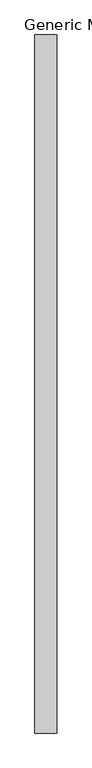
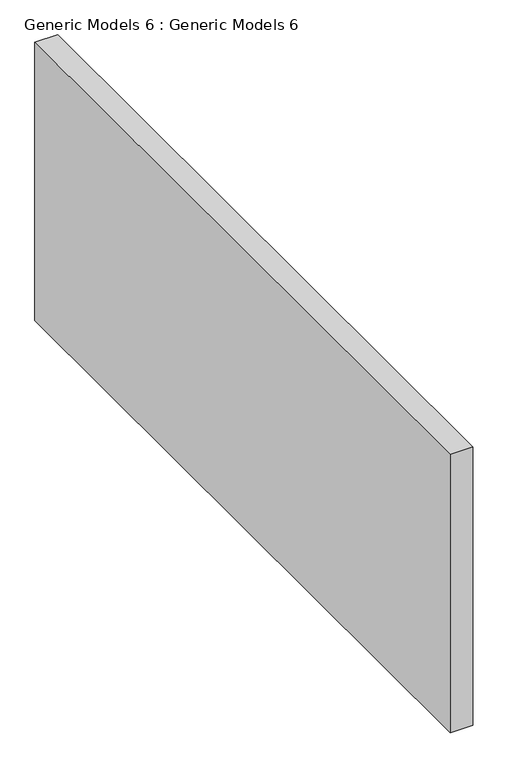
"""IFC4 building model written with IfcOpenShell, lengths in millimetres: proxy geometry, Generic Models 6 : Generic Models 6."""

from ifc_helpers import new_model, si_unit, frame, origin, place, context, project, spatial, polyline, outline, extrude, source, transform, mapped, element, save


def generic_models_6_generic_models_6_105658a1(model_context):
    return source(origin(), model_context, "Body", "SweptSolid", [
        extrude(outline(polyline([(-9814.7781265, -5997.1687648), (-9814.7781265, -4389.2142532), (-9763.9781265, -4389.2142532), (-9763.9781265, -5997.1687648), (-9814.7781265, -5997.1687648)])), frame((0.0, 0.0, 5791.2), z_axis=(0.0, 0.0, 1.0), x_axis=(1.0, 0.0, 0.0)), (0.0, 0.0, 1.0), 657.9042808),
    ])


if __name__ == "__main__":
    model = new_model("IFC4")
    model_context = context("Model", 3, world=origin())
    ifc_project = project(units=[si_unit("LENGTHUNIT", "METRE", prefix="MILLI")], contexts=[model_context])
    site = spatial("IfcSite", under=ifc_project)
    building = spatial("IfcBuilding", under=site)
    placement = place(None, origin())
    generic_models_6_generic_models_6_shape = generic_models_6_generic_models_6_105658a1(model_context)
    element("IfcBuildingElementProxy", 1, Name="Generic Models 6 : Generic Models 6", ObjectType="Generic Models 6 : Generic Models 6", at=placement, inside=building, context=model_context, shape_type="MappedRepresentation", body=[
        mapped(generic_models_6_generic_models_6_shape, transform((0.0, 0.0, 0.0), x_axis=(1.0, 0.0, 0.0), y_axis=(0.0, 1.0, 0.0), z_axis=(0.0, 0.0, 1.0))),
    ])
    save(model, "model.ifc")
